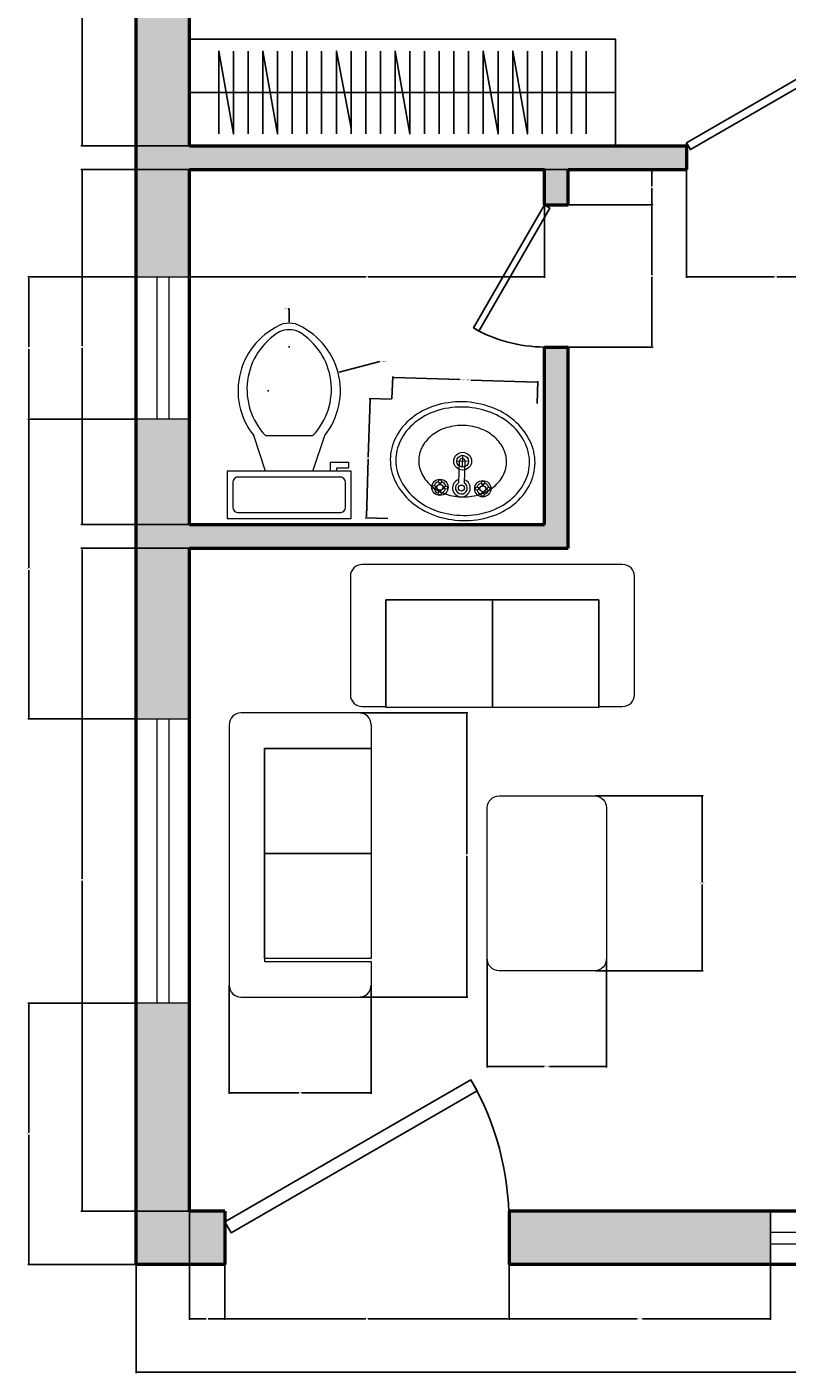
# Model space of a CAD drawing. Units: inches. Extents: x 2130 to 2425, y 2862 to 3216.
# Tile 1 of 4: x 2130 to 2259, y 2862 to 3089. Entities that reach past the tile are written whole.
import ezdxf

# ---------------------------------------------------------------- set-up
doc = ezdxf.new("R2010")
doc.units = ezdxf.units.IN
for name, color, linetype, lineweight in [('A-ANNO-DIMS', 2, 'Continuous', 18), ('A-DOOR', 3, 'Continuous', 25), ('A-FLOR-CASE', 9, 'Continuous', 25), ('A-FLOR-FIXT', 9, 'Continuous', 18), ('A-FURN', 8, 'Continuous', 18), ('A-GLAZ', 4, 'Continuous', 18), ('A-WALL', 7, 'Continuous', 50), ('A-WALL-PATT', 18, 'Continuous', 13)]:
    doc.layers.add(name, color=color, linetype=linetype, lineweight=lineweight)
doc.styles.get("Standard").update_dxf_attribs({"font": 'arial.ttf'})
doc.dimstyles.get("Standard").update_dxf_attribs({"dimtxt": 0.18, "dimasz": 0.18, "dimexe": 0.18, "dimexo": 0.0625, "dimgap": 0.09, "dimtad": 0, "dimtih": 1, "dimtoh": 1, "dimdec": 4, "dimzin": 0, "dimdsep": 46, "dimtxsty": 'Standard', "dimcen": 0.09, "dimadec": 0, "dimazin": 0, "dimtfac": 1, "dimtdec": 4, "dimtofl": 0, "dimtmove": 0, "dimatfit": 3, "dimfxl": 1, "dimtolj": 1, "dimtzin": 0, "dimarcsym": 0})

# ---------------------------------------------------------------- blocks, each defined once
blk = doc.blocks.new('Sink - Oval top')
for p, q in [((-1, 0), (1, 0)), ((0, 1), (0, -1))]:
    blk.add_line(p, q)
for points in [[(-12.23, 0.39, 0.117634), (-11.46, -3.36, 0.104469), (-8.88, -6.8, 0.090016), (-5.08, -9.07, 0.08192), (-0.32, -10.02, 0.08192), (4.49, -9.38, 0.090016), (8.42, -7.36, 0.104469), (11.22, -4.09, 0.117634), (12.23, -0.39, 0.117634), (11.46, 3.36, 0.104469), (8.88, 6.8, 0.090016), (5.08, 9.07, 0.08192), (0.32, 10.02, 0.08192), (-4.49, 9.38, 0.090016), (-8.42, 7.36, 0.104469), (-11.22, 4.09, 0.117634)], [(-11.29, 0.16, 0.118622), (-10.52, -3.25, 0.104678), (-8.07, -6.36, 0.089562), (-4.54, -8.37, 0.081185), (-0.13, -9.15, 0.081185), (4.3, -8.49, 0.089562), (7.89, -6.58, 0.104678), (10.42, -3.55, 0.118622), (11.29, -0.16, 0.118622), (10.52, 3.25, 0.104678), (8.07, 6.36, 0.089562), (4.54, 8.37, 0.081185), (0.13, 9.15, 0.081185), (-4.3, 8.49, 0.089562), (-7.89, 6.58, 0.104678), (-10.42, 3.55, 0.118622)], [(-7.42, 0.08, 0.118283), (-6.91, -2.17, 0.104607), (-5.29, -4.21, 0.089718), (-2.97, -5.53, 0.081436), (-0.07, -6.04, 0.081436), (2.84, -5.59, 0.089718), (5.2, -4.33, 0.104607), (6.86, -2.32, 0.118283), (7.42, -0.08, 0.118283), (6.91, 2.17, 0.104607), (5.29, 4.21, 0.089718), (2.97, 5.53, 0.081436), (0.07, 6.04, 0.081436), (-2.84, 5.59, 0.089718), (-5.2, 4.33, 0.104607), (-6.86, 2.32, 0.118283)]]:
    blk.add_lwpolyline(points, format="xyb", close=True)
for radius in [1.5, 1]:
    blk.add_circle((0, 0), radius)
blk = doc.blocks.new('Faucet - Bathroom top')
for p, q in [((-4.107, 0.125), (-4.375, 0.125)), ((-3.75, 0.4788), (-3.75, 0.75)), ((-3.5, 0.482), (-3.5, 0.75)), ((-3.1461, 0.125), (-2.875, 0.125)), ((3.143, 0.125), (2.875, 0.125)), ((3.5, 0.4788), (3.5, 0.75)), ((3.75, 0.482), (3.75, 0.75)), ((4.1039, 0.125), (4.375, 0.125)), ((-4.1039, -0.125), (-4.375, -0.125)), ((-3.75, -0.4821), (-3.75, -0.75)), ((-3.5, -0.4789), (-3.5, -0.75)), ((-3.143, -0.125), (-2.875, -0.125)), ((-0.5, -0.8639), (-0.5, -4.5)), ((0.5, -4.5), (0.5, -0.8631)), ((3.1461, -0.125), (2.875, -0.125)), ((3.5, -0.4821), (3.5, -0.75)), ((3.75, -0.4789), (3.75, -0.75)), ((4.107, -0.125), (4.375, -0.125))]:
    blk.add_line(p, q)
for centre, radius in [((-3.625, 0), 1.375), ((-4.625, 0), 0.2795), ((-3.625, 0), 0.5), ((-3.625, 1), 0.2795), ((-2.625, 0), 0.2795), ((0, 0), 0.5), ((3.625, 0), 1.375), ((2.625, 0), 0.2795), ((3.625, 0), 0.5), ((3.625, 1), 0.2795), ((4.625, 0), 0.2795), ((-3.625, -1), 0.2795), ((3.625, -1), 0.2795)]:
    blk.add_circle(centre, radius)
for centre, radius, start, end in [((-3.625, 0), 1, 105.2407, 164.2093), ((-3.625, 0), 1, 16.44125, 74.07887), ((0, 0), 1.5, 289.6514, 250.3603), ((0, 0), 1, 300.3431, 239.7554), ((3.625, 0), 1, 106.12, 164.0884), ((3.625, 0), 1, 16.23422, 73.90469), ((-3.625, 0), 1, 196.2342, 253.9047), ((-3.625, 0), 1, 286.12, 344.0884), ((3.625, 0), 1, 196.4413, 254.0789), ((3.625, 0), 1, 285.2407, 344.2093), ((0, -4.5), 0.5, 180, 0)]:
    blk.add_arc(centre, radius, start, end)
blk = doc.blocks.new('Toilet - top')
for p, q in [((9.5, -6), (9.5, -2)), ((-10, -8.5), (-8, -8.5)), ((-10, -9.5), (-10, -8.5)), ((-8, -8.5), (-8, -8)), ((-7, -8), (-7, -9.5)), ((-4, -8), (-6, -14)), ((4, -8), (6, -14)), ((-7, -9.5), (-10, -9.5)), ((4, -14), (-4, -14))]:
    blk.add_line(p, q)
blk.add_lwpolyline([(10.5, -8), (10.5, 0), (-10.5, 0), (-10.5, -8)], close=True)
for points in [[(-9.5, -2), (-9.5, -6)], [(8.5, -1), (-8.5, -1)], [(-8.5, -7), (8.5, -7)]]:
    blk.add_lwpolyline(points)
for centre, radius, start, end in [((-8.62, -1.88), 0.884, 81.8699, 188.1301), ((8.62, -1.88), 0.884, 351.8699, 98.1301), ((-8.62, -6.12), 0.884, 171.8699, 278.1301), ((8.62, -6.12), 0.884, 261.8699, 8.1301), ((3.52, -21.58), 12.17, 141.4691, 247.9714), ((4.2, -21.82), 11.33, 136.3677, 238.9468), ((-3.52, -21.58), 12.17, 292.0284, 38.5307), ((-4.2, -21.82), 11.33, 301.053, 43.6321), ((0, -27.88), 4, 245.7318, 294.2682), ((0, -29), 4, 254.8605, 285.1395)]:
    blk.add_arc(centre, radius, start, end)
blk = doc.blocks.new('*U10')
for p, q in [((0, 0), (0, -6)), ((40, 0), (40, -6))]:
    blk.add_line(p, q)
blk.add_lwpolyline([(0, 0), (34.64, 20), (35.52, 18.48), (0.87, -1.52)], close=True)
blk.add_arc((0, 0), 40, 0, 30)
blk = doc.blocks.new('*U11')
for p, q in [((0, 0), (0, 6)), ((40, 0), (40, 6))]:
    blk.add_line(p, q)
blk.add_lwpolyline([(0, 0), (34.64, -20), (35.52, -18.48), (0.87, 1.52)], close=True)
blk.add_arc((0, 0), 40, 330, 0)
blk = doc.blocks.new('WIN-48IN')
for p, q in [((0, 0), (0, 9)), ((48, 9), (48, 0)), ((0, 5.5), (48, 5.5)), ((0, 3.5), (48, 3.5))]:
    blk.add_line(p, q)
blk = doc.blocks.new('WARDROBE-72X18IN')
for p, q in [((0, 0), (0, 72)), ((0, 72), (18, 72)), ((9, 72), (9, 0)), ((18, 72), (18, 0)), ((2, 62.07), (16, 62.07)), ((2, 54.62), (16, 54.62)), ((2, 52.14), (16, 52.14)), ((2, 49.66), (16, 49.66)), ((2, 44.69), (16, 44.69)), ((2, 42.21), (16, 42.21)), ((2, 39.72), (16, 39.72)), ((2, 32.28), (16, 32.28)), ((2, 29.79), (16, 29.79)), ((2, 27.31), (16, 27.31)), ((2, 24.83), (16, 24.83)), ((2, 12.41), (16, 12.41)), ((2, 9.93), (16, 9.93)), ((2, 7.45), (16, 7.45)), ((2, 4.97), (16, 4.97)), ((18, 0), (0, 0))]:
    blk.add_line(p, q)
for points in [[(2, 67.03), (16, 67.03), (2, 64.55), (16, 64.55)], [(2, 59.59), (16, 59.59), (2, 57.1), (16, 57.1)], [(2, 47.17), (16, 47.17), (2.98, 44.69)], [(2, 37.24), (16, 37.24), (2, 34.76), (16, 34.76)], [(2, 22.35), (16, 22.35), (2, 19.86), (16, 19.86)], [(2, 17.38), (16, 17.38), (2, 14.9), (16, 14.9)]]:
    blk.add_lwpolyline(points)
blk.add_lwpolyline([(0, 0), (18, 0)], close=True)
blk = doc.blocks.new('*D23')
at = {"layer": 'A-ANNO-DIMS', "color": 0, "lineweight": -2, "transparency": 16777216}
for p, q in [((2191.77, 3026.18), (2191.89, 3029.98)), ((2192.07, 3029.8), (2203.22, 3029.44)), ((2216.25, 3029.02), (2205.09, 3029.38)), ((2216.31, 3025.39), (2216.43, 3029.19))]:
    blk.add_line(p, q, dxfattribs=at)
at = {"layer": 'A-ANNO-DIMS', "color": 0, "transparency": 16777216}
for points in [[(2192.07, 3029.83), (2192.07, 3029.77), (2191.89, 3029.8)], [(2216.25, 3029.05), (2216.24, 3028.99), (2216.43, 3029.01)]]:
    blk.add_solid(points, dxfattribs=at)
at = {"layer": 'Defpoints', "color": 0, "transparency": 16777216}
for p in [(2191.89, 3029.8), (2191.77, 3026.12), (2216.31, 3025.33)]:
    blk.add_point(p, dxfattribs=at)
at = {"layer": 'A-ANNO-DIMS', "color": 0, "transparency": 16777216, "insert": (2204.16, 3029.41), "char_height": 0.18, "attachment_point": 5}
blk.add_mtext('\\A1;BASIN 25 TYP.', dxfattribs=at)
blk = doc.blocks.new('*D24')
at = {"layer": 'A-ANNO-DIMS', "color": 0, "lineweight": -2, "transparency": 16777216}
for p, q in [((2188.08, 3026.06), (2187.77, 3016.36)), ((2191.71, 3026.12), (2187.91, 3026.25)), ((2187.45, 3006.29), (2187.76, 3015.99)), ((2191.06, 3006), (2187.26, 3006.12))]:
    blk.add_line(p, q, dxfattribs=at)
at = {"layer": 'A-ANNO-DIMS', "color": 0, "transparency": 16777216}
for points in [[(2188.05, 3026.06), (2188.11, 3026.06), (2188.09, 3026.24)], [(2187.42, 3006.29), (2187.48, 3006.29), (2187.44, 3006.11)]]:
    blk.add_solid(points, dxfattribs=at)
at = {"layer": 'Defpoints', "color": 0, "transparency": 16777216}
for p in [(2191.77, 3026.12), (2187.44, 3006.11), (2191.12, 3006)]:
    blk.add_point(p, dxfattribs=at)
at = {"layer": 'A-ANNO-DIMS', "color": 0, "transparency": 16777216, "insert": (2187.76, 3016.18), "char_height": 0.18, "attachment_point": 5}
blk.add_mtext('\\A1;20 TYP.', dxfattribs=at)
blk = doc.blocks.new('*D35')
at = {"layer": 'A-ANNO-DIMS', "color": 0, "lineweight": -2, "transparency": 16777216}
for p, q in [((2148.55, 2879.89), (2148.55, 2861.62)), ((2406.55, 2879.89), (2406.55, 2861.62)), ((2148.73, 2861.8), (2277.26, 2861.8)), ((2406.37, 2861.8), (2277.84, 2861.8))]:
    blk.add_line(p, q, dxfattribs=at)
at = {"layer": 'A-ANNO-DIMS', "color": 0, "transparency": 16777216}
for points in [[(2148.73, 2861.83), (2148.73, 2861.77), (2148.55, 2861.8)], [(2406.37, 2861.83), (2406.37, 2861.77), (2406.55, 2861.8)]]:
    blk.add_solid(points, dxfattribs=at)
at = {"layer": 'Defpoints', "color": 0, "transparency": 16777216}
for p in [(2148.55, 2879.95), (2406.55, 2879.95), (2406.55, 2861.8)]:
    blk.add_point(p, dxfattribs=at)
at = {"layer": 'A-ANNO-DIMS', "color": 0, "transparency": 16777216, "insert": (2277.55, 2861.8), "char_height": 0.18, "attachment_point": 5}
blk.add_mtext('\\A1;258', dxfattribs=at)
blk = doc.blocks.new('*D39')
at = {"layer": 'A-ANNO-DIMS', "color": 0, "lineweight": -2, "transparency": 16777216}
for p, q in [((2157.55, 2888.89), (2157.55, 2870.62)), ((2163.55, 2888.89), (2163.55, 2870.62)), ((2157.73, 2870.8), (2160.4, 2870.8)), ((2163.37, 2870.8), (2160.7, 2870.8))]:
    blk.add_line(p, q, dxfattribs=at)
at = {"layer": 'A-ANNO-DIMS', "color": 0, "transparency": 16777216}
for points in [[(2157.73, 2870.83), (2157.73, 2870.77), (2157.55, 2870.8)], [(2163.37, 2870.83), (2163.37, 2870.77), (2163.55, 2870.8)]]:
    blk.add_solid(points, dxfattribs=at)
at = {"layer": 'Defpoints', "color": 0, "transparency": 16777216}
for p in [(2157.55, 2888.95), (2163.55, 2888.95), (2157.55, 2870.8)]:
    blk.add_point(p, dxfattribs=at)
at = {"layer": 'A-ANNO-DIMS', "color": 0, "transparency": 16777216, "insert": (2160.55, 2870.8), "char_height": 0.18, "attachment_point": 5}
blk.add_mtext('\\A1;6', dxfattribs=at)
blk = doc.blocks.new('*D40')
at = {"layer": 'A-ANNO-DIMS', "color": 0, "lineweight": -2, "transparency": 16777216}
for p, q in [((2163.55, 2888.89), (2163.55, 2870.62)), ((2211.55, 2888.89), (2211.55, 2870.62)), ((2163.73, 2870.8), (2187.33, 2870.8)), ((2211.37, 2870.8), (2187.77, 2870.8))]:
    blk.add_line(p, q, dxfattribs=at)
at = {"layer": 'A-ANNO-DIMS', "color": 0, "transparency": 16777216}
for points in [[(2163.73, 2870.83), (2163.73, 2870.77), (2163.55, 2870.8)], [(2211.37, 2870.83), (2211.37, 2870.77), (2211.55, 2870.8)]]:
    blk.add_solid(points, dxfattribs=at)
at = {"layer": 'Defpoints', "color": 0, "transparency": 16777216}
for p in [(2163.55, 2888.95), (2211.55, 2888.95), (2163.55, 2870.8)]:
    blk.add_point(p, dxfattribs=at)
at = {"layer": 'A-ANNO-DIMS', "color": 0, "transparency": 16777216, "insert": (2187.55, 2870.8), "char_height": 0.18, "attachment_point": 5}
blk.add_mtext('\\A1;48', dxfattribs=at)
blk = doc.blocks.new('*D41')
at = {"layer": 'A-ANNO-DIMS', "color": 0, "lineweight": -2, "transparency": 16777216}
for p, q in [((2211.55, 2888.89), (2211.55, 2870.62)), ((2255.75, 2888.89), (2255.75, 2870.62)), ((2211.73, 2870.8), (2233.18, 2870.8)), ((2255.57, 2870.8), (2234.12, 2870.8))]:
    blk.add_line(p, q, dxfattribs=at)
at = {"layer": 'A-ANNO-DIMS', "color": 0, "transparency": 16777216}
for points in [[(2211.73, 2870.83), (2211.73, 2870.77), (2211.55, 2870.8)], [(2255.57, 2870.83), (2255.57, 2870.77), (2255.75, 2870.8)]]:
    blk.add_solid(points, dxfattribs=at)
at = {"layer": 'Defpoints', "color": 0, "transparency": 16777216}
for p in [(2211.55, 2888.95), (2255.75, 2888.95), (2211.55, 2870.8)]:
    blk.add_point(p, dxfattribs=at)
at = {"layer": 'A-ANNO-DIMS', "color": 0, "transparency": 16777216, "insert": (2233.65, 2870.8), "char_height": 0.18, "attachment_point": 5}
blk.add_mtext('\\A1;44.195', dxfattribs=at)
blk = doc.blocks.new('*D43')
at = {"layer": 'A-ANNO-DIMS', "color": 0, "lineweight": -2, "transparency": 16777216}
for p, q in [((2148.49, 2924.14), (2130.22, 2924.14)), ((2130.4, 2923.96), (2130.4, 2902.23)), ((2130.4, 2880.13), (2130.4, 2901.86)), ((2148.49, 2879.95), (2130.22, 2879.95))]:
    blk.add_line(p, q, dxfattribs=at)
at = {"layer": 'A-ANNO-DIMS', "color": 0, "transparency": 16777216}
for points in [[(2130.37, 2923.96), (2130.43, 2923.96), (2130.4, 2924.14)], [(2130.37, 2880.13), (2130.43, 2880.13), (2130.4, 2879.95)]]:
    blk.add_solid(points, dxfattribs=at)
at = {"layer": 'Defpoints', "color": 0, "transparency": 16777216}
for p in [(2130.4, 2924.14), (2148.55, 2924.14), (2148.55, 2879.95)]:
    blk.add_point(p, dxfattribs=at)
at = {"layer": 'A-ANNO-DIMS', "color": 0, "transparency": 16777216, "insert": (2130.4, 2902.05), "char_height": 0.18, "attachment_point": 5}
blk.add_mtext('\\A1;44.18', dxfattribs=at)
blk = doc.blocks.new('*D44')
at = {"layer": 'A-ANNO-DIMS', "color": 0, "lineweight": -2, "transparency": 16777216}
for p, q in [((2148.49, 3022.79), (2130.22, 3022.79)), ((2130.4, 3022.61), (2130.4, 2997.65)), ((2130.4, 2972.32), (2130.4, 2997.28)), ((2148.49, 2972.14), (2130.22, 2972.14))]:
    blk.add_line(p, q, dxfattribs=at)
at = {"layer": 'A-ANNO-DIMS', "color": 0, "transparency": 16777216}
for points in [[(2130.37, 3022.61), (2130.43, 3022.61), (2130.4, 3022.79)], [(2130.37, 2972.32), (2130.43, 2972.32), (2130.4, 2972.14)]]:
    blk.add_solid(points, dxfattribs=at)
at = {"layer": 'Defpoints', "color": 0, "transparency": 16777216}
for p in [(2130.4, 3022.79), (2148.55, 3022.79), (2148.55, 2972.14)]:
    blk.add_point(p, dxfattribs=at)
at = {"layer": 'A-ANNO-DIMS', "color": 0, "transparency": 16777216, "insert": (2130.4, 2997.46), "char_height": 0.18, "attachment_point": 5}
blk.add_mtext('\\A1;50.65', dxfattribs=at)
blk = doc.blocks.new('*D45')
at = {"layer": 'A-ANNO-DIMS', "color": 0, "lineweight": -2, "transparency": 16777216}
for p, q in [((2148.49, 3046.79), (2130.22, 3046.79)), ((2130.4, 3046.61), (2130.4, 3034.97)), ((2130.4, 3022.97), (2130.4, 3034.61)), ((2148.49, 3022.79), (2130.22, 3022.79))]:
    blk.add_line(p, q, dxfattribs=at)
at = {"layer": 'A-ANNO-DIMS', "color": 0, "transparency": 16777216}
for points in [[(2130.37, 3046.61), (2130.43, 3046.61), (2130.4, 3046.79)], [(2130.37, 3022.97), (2130.43, 3022.97), (2130.4, 3022.79)]]:
    blk.add_solid(points, dxfattribs=at)
at = {"layer": 'Defpoints', "color": 0, "transparency": 16777216}
for p in [(2130.4, 3046.79), (2148.55, 3046.79), (2148.55, 3022.79)]:
    blk.add_point(p, dxfattribs=at)
at = {"layer": 'A-ANNO-DIMS', "color": 0, "transparency": 16777216, "insert": (2130.4, 3034.79), "char_height": 0.18, "attachment_point": 5}
blk.add_mtext('\\A1;24', dxfattribs=at)
blk = doc.blocks.new('*D49')
at = {"layer": 'A-ANNO-DIMS', "color": 0, "lineweight": -2, "transparency": 16777216}
for p, q in [((2157.49, 3188.95), (2139.22, 3188.95)), ((2139.4, 3188.77), (2139.4, 3129.14)), ((2139.4, 3069.13), (2139.4, 3128.77)), ((2157.49, 3068.95), (2139.22, 3068.95))]:
    blk.add_line(p, q, dxfattribs=at)
at = {"layer": 'A-ANNO-DIMS', "color": 0, "transparency": 16777216}
for points in [[(2139.37, 3188.77), (2139.43, 3188.77), (2139.4, 3188.95)], [(2139.37, 3069.13), (2139.43, 3069.13), (2139.4, 3068.95)]]:
    blk.add_solid(points, dxfattribs=at)
at = {"layer": 'Defpoints', "color": 0, "transparency": 16777216}
for p in [(2139.4, 3188.95), (2157.55, 3188.95), (2157.55, 3068.95)]:
    blk.add_point(p, dxfattribs=at)
at = {"layer": 'A-ANNO-DIMS', "color": 0, "transparency": 16777216, "insert": (2139.4, 3128.95), "char_height": 0.18, "attachment_point": 5}
blk.add_mtext('\\A1;120', dxfattribs=at)
blk = doc.blocks.new('*D50')
at = {"layer": 'A-ANNO-DIMS', "color": 0, "lineweight": -2, "transparency": 16777216}
for p, q in [((2157.55, 3064.89), (2157.55, 3046.62)), ((2217.55, 3064.89), (2217.55, 3046.62)), ((2157.73, 3046.8), (2187.33, 3046.8)), ((2217.37, 3046.8), (2187.77, 3046.8))]:
    blk.add_line(p, q, dxfattribs=at)
at = {"layer": 'A-ANNO-DIMS', "color": 0, "transparency": 16777216}
for points in [[(2157.73, 3046.83), (2157.73, 3046.77), (2157.55, 3046.8)], [(2217.37, 3046.83), (2217.37, 3046.77), (2217.55, 3046.8)]]:
    blk.add_solid(points, dxfattribs=at)
at = {"layer": 'Defpoints', "color": 0, "transparency": 16777216}
for p in [(2157.55, 3064.95), (2217.55, 3064.95), (2157.55, 3046.8)]:
    blk.add_point(p, dxfattribs=at)
at = {"layer": 'A-ANNO-DIMS', "color": 0, "transparency": 16777216, "insert": (2187.55, 3046.8), "char_height": 0.18, "attachment_point": 5}
blk.add_mtext('\\A1;60', dxfattribs=at)
blk = doc.blocks.new('*D51')
at = {"layer": 'A-ANNO-DIMS', "color": 0, "lineweight": -2, "transparency": 16777216}
for p, q in [((2157.49, 3064.95), (2139.22, 3064.95)), ((2139.4, 3064.77), (2139.4, 3035.14)), ((2139.4, 3005.13), (2139.4, 3034.77)), ((2157.49, 3004.95), (2139.22, 3004.95))]:
    blk.add_line(p, q, dxfattribs=at)
at = {"layer": 'A-ANNO-DIMS', "color": 0, "transparency": 16777216}
for points in [[(2139.37, 3064.77), (2139.43, 3064.77), (2139.4, 3064.95)], [(2139.37, 3005.13), (2139.43, 3005.13), (2139.4, 3004.95)]]:
    blk.add_solid(points, dxfattribs=at)
at = {"layer": 'Defpoints', "color": 0, "transparency": 16777216}
for p in [(2139.4, 3064.95), (2157.55, 3064.95), (2157.55, 3004.95)]:
    blk.add_point(p, dxfattribs=at)
at = {"layer": 'A-ANNO-DIMS', "color": 0, "transparency": 16777216, "insert": (2139.4, 3034.95), "char_height": 0.18, "attachment_point": 5}
blk.add_mtext('\\A1;60', dxfattribs=at)
blk = doc.blocks.new('*D52')
at = {"layer": 'A-ANNO-DIMS', "color": 0, "lineweight": -2, "transparency": 16777216}
for p, q in [((2157.49, 3000.95), (2139.22, 3000.95)), ((2139.4, 3000.77), (2139.4, 2945.13)), ((2139.4, 2889.13), (2139.4, 2944.77)), ((2157.49, 2888.95), (2139.22, 2888.95))]:
    blk.add_line(p, q, dxfattribs=at)
at = {"layer": 'A-ANNO-DIMS', "color": 0, "transparency": 16777216}
for points in [[(2139.37, 3000.77), (2139.43, 3000.77), (2139.4, 3000.95)], [(2139.37, 2889.13), (2139.43, 2889.13), (2139.4, 2888.95)]]:
    blk.add_solid(points, dxfattribs=at)
at = {"layer": 'Defpoints', "color": 0, "transparency": 16777216}
for p in [(2139.4, 3000.95), (2157.55, 3000.95), (2157.55, 2888.95)]:
    blk.add_point(p, dxfattribs=at)
at = {"layer": 'A-ANNO-DIMS', "color": 0, "transparency": 16777216, "insert": (2139.4, 2944.95), "char_height": 0.18, "attachment_point": 5}
blk.add_mtext('\\A1;112', dxfattribs=at)
blk = doc.blocks.new('*D57')
at = {"layer": 'A-ANNO-DIMS', "color": 0, "lineweight": -2, "transparency": 16777216}
for p, q in [((2241.55, 3064.89), (2241.55, 3046.62)), ((2271.55, 3064.89), (2271.55, 3046.62)), ((2241.73, 3046.8), (2256.33, 3046.8)), ((2271.37, 3046.8), (2256.77, 3046.8))]:
    blk.add_line(p, q, dxfattribs=at)
at = {"layer": 'A-ANNO-DIMS', "color": 0, "transparency": 16777216}
for points in [[(2241.73, 3046.83), (2241.73, 3046.77), (2241.55, 3046.8)], [(2271.37, 3046.83), (2271.37, 3046.77), (2271.55, 3046.8)]]:
    blk.add_solid(points, dxfattribs=at)
at = {"layer": 'Defpoints', "color": 0, "transparency": 16777216}
for p in [(2241.55, 3064.95), (2271.55, 3064.95), (2241.55, 3046.8)]:
    blk.add_point(p, dxfattribs=at)
at = {"layer": 'A-ANNO-DIMS', "color": 0, "transparency": 16777216, "insert": (2256.55, 3046.8), "char_height": 0.18, "attachment_point": 5}
blk.add_mtext('\\A1;30', dxfattribs=at)
blk = doc.blocks.new('*D61')
at = {"layer": 'A-ANNO-DIMS', "color": 0, "lineweight": -2, "transparency": 16777216}
for p, q in [((2217.61, 3058.95), (2235.88, 3058.95)), ((2235.7, 3058.77), (2235.7, 3047.13)), ((2235.7, 3035.13), (2235.7, 3046.77)), ((2217.61, 3034.95), (2235.88, 3034.95))]:
    blk.add_line(p, q, dxfattribs=at)
at = {"layer": 'A-ANNO-DIMS', "color": 0, "transparency": 16777216}
for points in [[(2235.67, 3058.77), (2235.73, 3058.77), (2235.7, 3058.95)], [(2235.67, 3035.13), (2235.73, 3035.13), (2235.7, 3034.95)]]:
    blk.add_solid(points, dxfattribs=at)
at = {"layer": 'Defpoints', "color": 0, "transparency": 16777216}
for p in [(2217.55, 3058.95), (2217.55, 3034.95), (2235.7, 3034.95)]:
    blk.add_point(p, dxfattribs=at)
at = {"layer": 'A-ANNO-DIMS', "color": 0, "transparency": 16777216, "insert": (2235.7, 3046.95), "char_height": 0.18, "attachment_point": 5}
blk.add_mtext('\\A1;24', dxfattribs=at)
blk = doc.blocks.new('*D62')
at = {"layer": 'A-ANNO-DIMS', "color": 0, "lineweight": -2, "transparency": 16777216}
for p, q in [((2217.61, 3064.95), (2235.88, 3064.95)), ((2235.7, 3064.77), (2235.7, 3062.14)), ((2235.7, 3059.13), (2235.7, 3061.77)), ((2217.61, 3058.95), (2235.88, 3058.95))]:
    blk.add_line(p, q, dxfattribs=at)
at = {"layer": 'A-ANNO-DIMS', "color": 0, "transparency": 16777216}
for points in [[(2235.67, 3064.77), (2235.73, 3064.77), (2235.7, 3064.95)], [(2235.67, 3059.13), (2235.73, 3059.13), (2235.7, 3058.95)]]:
    blk.add_solid(points, dxfattribs=at)
at = {"layer": 'Defpoints', "color": 0, "transparency": 16777216}
for p in [(2217.55, 3064.95), (2217.55, 3058.95), (2235.7, 3058.95)]:
    blk.add_point(p, dxfattribs=at)
at = {"layer": 'A-ANNO-DIMS', "color": 0, "transparency": 16777216, "insert": (2235.7, 3061.95), "char_height": 0.18, "attachment_point": 5}
blk.add_mtext('\\A1;6', dxfattribs=at)
blk = doc.blocks.new('*D67')
at = {"layer": 'A-ANNO-DIMS', "color": 0, "lineweight": -2, "transparency": 16777216}
for p, q in [((2186.32, 2973.14), (2204.59, 2973.14)), ((2204.41, 2972.96), (2204.41, 2949.33)), ((2204.41, 2925.32), (2204.41, 2948.96)), ((2186.32, 2925.14), (2204.59, 2925.14))]:
    blk.add_line(p, q, dxfattribs=at)
at = {"layer": 'A-ANNO-DIMS', "color": 0, "transparency": 16777216}
for points in [[(2204.38, 2972.96), (2204.44, 2972.96), (2204.41, 2973.14)], [(2204.38, 2925.32), (2204.44, 2925.32), (2204.41, 2925.14)]]:
    blk.add_solid(points, dxfattribs=at)
at = {"layer": 'Defpoints', "color": 0, "transparency": 16777216}
for p in [(2186.26, 2973.14), (2186.26, 2925.14), (2204.41, 2925.14)]:
    blk.add_point(p, dxfattribs=at)
at = {"layer": 'A-ANNO-DIMS', "color": 0, "transparency": 16777216, "insert": (2204.41, 2949.14), "char_height": 0.18, "attachment_point": 5}
blk.add_mtext('\\A1;48', dxfattribs=at)
blk = doc.blocks.new('*D68')
at = {"layer": 'A-ANNO-DIMS', "color": 0, "lineweight": -2, "transparency": 16777216}
for p, q in [((2164.26, 2927.08), (2164.26, 2908.81)), ((2188.26, 2927.08), (2188.26, 2908.81)), ((2164.44, 2908.99), (2176.04, 2908.99)), ((2188.08, 2908.99), (2176.48, 2908.99))]:
    blk.add_line(p, q, dxfattribs=at)
at = {"layer": 'A-ANNO-DIMS', "color": 0, "transparency": 16777216}
for points in [[(2164.44, 2909.02), (2164.44, 2908.96), (2164.26, 2908.99)], [(2188.08, 2909.02), (2188.08, 2908.96), (2188.26, 2908.99)]]:
    blk.add_solid(points, dxfattribs=at)
at = {"layer": 'Defpoints', "color": 0, "transparency": 16777216}
for p in [(2164.26, 2927.14), (2188.26, 2927.14), (2164.26, 2908.99)]:
    blk.add_point(p, dxfattribs=at)
at = {"layer": 'A-ANNO-DIMS', "color": 0, "transparency": 16777216, "insert": (2176.26, 2908.99), "char_height": 0.18, "attachment_point": 5}
blk.add_mtext('\\A1;24', dxfattribs=at)
blk = doc.blocks.new('*D69')
at = {"layer": 'A-ANNO-DIMS', "color": 0, "lineweight": -2, "transparency": 16777216}
for p, q in [((2207.87, 2931.53), (2207.87, 2913.26)), ((2228.02, 2931.53), (2228.02, 2913.26)), ((2208.05, 2913.44), (2217.48, 2913.44)), ((2227.84, 2913.44), (2218.41, 2913.44))]:
    blk.add_line(p, q, dxfattribs=at)
at = {"layer": 'A-ANNO-DIMS', "color": 0, "transparency": 16777216}
for points in [[(2208.05, 2913.47), (2208.05, 2913.41), (2207.87, 2913.44)], [(2227.84, 2913.47), (2227.84, 2913.41), (2228.02, 2913.44)]]:
    blk.add_solid(points, dxfattribs=at)
at = {"layer": 'Defpoints', "color": 0, "transparency": 16777216}
for p in [(2207.87, 2931.59), (2228.02, 2931.59), (2207.87, 2913.44)]:
    blk.add_point(p, dxfattribs=at)
at = {"layer": 'A-ANNO-DIMS', "color": 0, "transparency": 16777216, "insert": (2217.94, 2913.44), "char_height": 0.18, "attachment_point": 5}
blk.add_mtext('\\A1;20.148', dxfattribs=at)
blk = doc.blocks.new('*D70')
at = {"layer": 'A-ANNO-DIMS', "color": 0, "lineweight": -2, "transparency": 16777216}
for p, q in [((2226.08, 2959.13), (2244.35, 2959.13)), ((2244.17, 2958.95), (2244.17, 2944.54)), ((2244.17, 2929.77), (2244.17, 2944.18)), ((2226.08, 2929.59), (2244.35, 2929.59))]:
    blk.add_line(p, q, dxfattribs=at)
at = {"layer": 'A-ANNO-DIMS', "color": 0, "transparency": 16777216}
for points in [[(2244.14, 2958.95), (2244.2, 2958.95), (2244.17, 2959.13)], [(2244.14, 2929.77), (2244.2, 2929.77), (2244.17, 2929.59)]]:
    blk.add_solid(points, dxfattribs=at)
at = {"layer": 'Defpoints', "color": 0, "transparency": 16777216}
for p in [(2226.02, 2959.13), (2226.02, 2929.59), (2244.17, 2929.59)]:
    blk.add_point(p, dxfattribs=at)
at = {"layer": 'A-ANNO-DIMS', "color": 0, "transparency": 16777216, "insert": (2244.17, 2944.36), "char_height": 0.18, "attachment_point": 5}
blk.add_mtext('\\A1;29.535', dxfattribs=at)
blk = doc.blocks.new('*D74')
at = {"layer": 'A-ANNO-DIMS', "color": 0, "lineweight": -2, "transparency": 16777216}
for p, q in [((2189.72, 3032.52), (2182.83, 3030.71)), ((2170.79, 3027.57), (2170.97, 3027.57)), ((2170.88, 3027.48), (2170.88, 3027.66))]:
    blk.add_line(p, q, dxfattribs=at)
at = {"layer": 'A-ANNO-DIMS', "color": 0, "transparency": 16777216}
blk.add_solid([(2182.82, 3030.73), (2182.84, 3030.68), (2182.65, 3030.66)], dxfattribs=at)
at = {"layer": 'Defpoints', "color": 0, "transparency": 16777216}
for p in [(2182.65, 3030.66), (2170.88, 3027.57)]:
    blk.add_point(p, dxfattribs=at)
at = {"layer": 'A-ANNO-DIMS', "color": 0, "transparency": 16777216, "insert": (2190.39, 3032.52), "char_height": 0.18, "attachment_point": 5}
blk.add_mtext('\\A1;4X R12.17', dxfattribs=at)
blk = doc.blocks.new('*D76')
at = {"layer": 'A-ANNO-DIMS', "color": 0, "lineweight": -2, "transparency": 16777216}
for p, q in [((2174.22, 3041.39), (2174.4, 3041.39)), ((2174.4, 3041.39), (2174.4, 3039.17)), ((2174.31, 3034.99), (2174.49, 3034.99)), ((2174.4, 3034.9), (2174.4, 3035.08))]:
    blk.add_line(p, q, dxfattribs=at)
at = {"layer": 'A-ANNO-DIMS', "color": 0, "transparency": 16777216}
blk.add_solid([(2174.43, 3039.17), (2174.37, 3039.17), (2174.4, 3038.99)], dxfattribs=at)
at = {"layer": 'Defpoints', "color": 0, "transparency": 16777216}
for p in [(2174.4, 3038.99), (2174.4, 3034.99)]:
    blk.add_point(p, dxfattribs=at)
at = {"layer": 'A-ANNO-DIMS', "color": 0, "transparency": 16777216, "insert": (2173.79, 3041.39), "char_height": 0.18, "attachment_point": 5}
blk.add_mtext('\\A1;4X R4', dxfattribs=at)

msp = doc.modelspace()

# ---------------------------------------------------------------- hatches: boundary and pattern name
at = {"layer": 'A-WALL-PATT'}
h = msp.add_hatch(color=256, dxfattribs=at)
h.dxf.hatch_style = 1
h.paths.add_polyline_path([(2186.3228, 3197.9544), (2148.5502, 3197.9544), (2148.5502, 3046.791), (2157.5502, 3046.791), (2157.5502, 3064.9544), (2217.5502, 3064.9544), (2217.5502, 3058.9544), (2221.1502, 3058.9544), (2221.5502, 3058.9544), (2221.5502, 3064.9544), (2241.5502, 3064.9544), (2241.5502, 3068.9544), (2157.5502, 3068.9544), (2157.5502, 3086.9544), (2157.5502, 3188.9544), (2186.3228, 3188.9544)])
h = msp.add_hatch(color=256, dxfattribs=at)
h.dxf.hatch_style = 1
h.paths.add_polyline_path([(2221.5502, 3034.9544), (2217.5502, 3034.9544), (2217.5502, 3004.9544), (2157.5502, 3004.9544), (2157.5502, 3022.791), (2148.5502, 3022.791), (2148.5502, 2972.1386), (2157.5502, 2972.1386), (2157.5502, 3000.9544), (2221.5502, 3000.9544)])
h = msp.add_hatch(color=256, dxfattribs=at)
h.dxf.hatch_style = 1
h.paths.add_polyline_path([(2163.5502, 2887.1544), (2163.5502, 2888.9544), (2157.5502, 2888.9544), (2157.5502, 2924.1386), (2148.5502, 2924.1386), (2148.5502, 2879.9544), (2163.5502, 2879.9544)])
h = msp.add_hatch(color=256, dxfattribs=at)
h.dxf.hatch_style = 1
h.paths.add_polyline_path([(2255.7452, 2888.9544), (2211.5502, 2888.9544), (2211.5502, 2879.9544), (2255.7452, 2879.9544)])

# ---------------------------------------------------------------- linework, layer by layer
at = {"layer": 'A-FURN'}
for p, q in [((2230.7457, 2998.2192), (2186.7457, 2998.2192)), ((2184.7457, 2996.2192), (2184.7457, 2976.2192)), ((2232.7457, 2976.2192), (2232.7457, 2996.2192)), ((2190.7457, 2992.2192), (2190.7457, 2974.2192)), ((2226.7457, 2992.2192), (2190.7457, 2992.2192)), ((2226.7457, 2974.2192), (2226.7457, 2992.2192)), ((2186.2568, 2973.1449), (2166.2568, 2973.1449)), ((2186.7457, 2974.2192), (2190.7457, 2974.2192)), ((2226.7457, 2974.2192), (2230.7457, 2974.2192)), ((2164.2568, 2971.1449), (2164.2568, 2927.1449)), ((2188.2568, 2971.1449), (2188.2568, 2967.1449)), ((2188.2568, 2967.1449), (2170.2568, 2967.1449)), ((2170.2568, 2967.1449), (2170.2568, 2931.1449)), ((2170.2568, 2931.1449), (2188.2568, 2931.1449)), ((2188.2568, 2931.1449), (2188.2568, 2927.1449)), ((2166.2568, 2925.1449), (2186.2568, 2925.1449))]:
    msp.add_line(p, q, dxfattribs=at)
for points in [[(2190.7457, 2992.2192), (2208.7457, 2992.2192), (2208.7457, 2974.0728), (2190.7457, 2974.0728)], [(2208.7457, 2992.2192), (2226.7457, 2992.2192), (2226.7457, 2974.0728), (2208.7457, 2974.0728)], [(2170.2568, 2967.1449), (2188.2568, 2967.1449), (2188.2568, 2949.3941), (2170.2568, 2949.3941)], [(2170.2568, 2949.3941), (2188.2568, 2949.3941), (2188.2568, 2931.6433), (2170.2568, 2931.6433)]]:
    msp.add_lwpolyline(points, close=True, dxfattribs=at)
msp.add_lwpolyline([(2209.8678, 2959.1295), (2226.0156, 2959.1295, -0.41421356), (2228.0156, 2957.1295), (2228.0156, 2931.5948, -0.41421356), (2226.0156, 2929.5948), (2209.8678, 2929.5948, -0.41421356), (2207.8678, 2931.5948), (2207.8678, 2957.1295, -0.41421356)], format="xyb", close=True, dxfattribs=at)
for centre, start, end in [((2186.7457, 2996.2192), 90, 180), ((2230.7457, 2996.2192), 0, 90), ((2186.7457, 2976.2192), 180, 270), ((2230.7457, 2976.2192), 270, 0), ((2166.2568, 2971.1449), 90, 180), ((2186.2568, 2971.1449), 0, 90), ((2166.2568, 2927.1449), 180, 270), ((2186.2568, 2927.1449), 270, 0)]:
    msp.add_arc(centre, 2, start, end, dxfattribs=at)
at = {"layer": 'A-GLAZ'}
for p, q in [((2148.5502, 3046.791), (2157.5502, 3046.791)), ((2152.0502, 3046.791), (2152.0502, 3022.791)), ((2154.0502, 3046.791), (2154.0502, 3022.791)), ((2157.5502, 3022.791), (2148.5502, 3022.791))]:
    msp.add_line(p, q, dxfattribs=at)
at = {"layer": 'A-WALL'}
for p, q in [((2157.5502, 3068.9544), (2157.5502, 3188.9544)), ((2157.5502, 3068.9544), (2241.5502, 3068.9544)), ((2241.5502, 3068.9544), (2241.5502, 3064.9544)), ((2157.5502, 3064.9544), (2217.5502, 3064.9544)), ((2157.5502, 3004.9544), (2157.5502, 3064.9544)), ((2217.5502, 3058.9544), (2217.5502, 3064.9544)), ((2221.5502, 3064.9544), (2241.5502, 3064.9544)), ((2221.5502, 3058.9544), (2221.5502, 3064.9544)), ((2217.5502, 3058.9544), (2221.5502, 3058.9544)), ((2217.5502, 3004.9544), (2217.5502, 3034.9544)), ((2217.5502, 3034.9544), (2221.5502, 3034.9544)), ((2221.5502, 3000.9544), (2221.5502, 3034.9544)), ((2157.5502, 3004.9544), (2217.5502, 3004.9544)), ((2157.5502, 2888.9544), (2157.5502, 3000.9544)), ((2157.5502, 3000.9544), (2221.5502, 3000.9544)), ((2163.5502, 2888.9544), (2157.5502, 2888.9544)), ((2163.5502, 2888.9544), (2163.5502, 2879.9544)), ((2323.5502, 2888.9544), (2211.5502, 2888.9544)), ((2211.5502, 2888.9544), (2211.5502, 2879.9544))]:
    msp.add_line(p, q, dxfattribs=at)
msp.add_lwpolyline([(2163.5502, 2879.9544), (2148.5502, 2879.9544), (2148.5502, 3197.9544), (2406.5502, 3197.9544), (2406.5502, 2879.9544), (2211.5502, 2879.9544)], dxfattribs=at)

# ---------------------------------------------------------------- block references
at = {"layer": 'A-DOOR'}
for p, xscale, yscale, zscale in [((2241.5502, 3069.4544), 0.75, 0.75, 0.75), ((2163.5502, 2887.1544), 1.199999999999999, 1.199999999999999, 1.199999999999999)]:
    msp.add_blockref('*U10', p, dxfattribs=dict(at, xscale=xscale, yscale=yscale, zscale=zscale))
at = {"layer": 'A-DOOR', "xscale": 0.6, "yscale": 0.6, "zscale": 0.6, "rotation": 270}
msp.add_blockref('*U11', (2217.5502, 3058.9544), dxfattribs=at)
at = {"layer": 'A-FLOR-CASE', "rotation": 90.0000000000085}
msp.add_blockref('WARDROBE-72X18IN', (2229.5506, 3068.9542), dxfattribs=at)
at = {"layer": 'A-FLOR-FIXT'}
for name, p, rotation in [('Toilet - top', (2174.4045, 3005.9873), 180), ('Sink - Oval top', (2203.7134, 3015.6629), 178.1544699151333), ('Faucet - Bathroom top', (2203.4996, 3011.1306), 178.1544699151333)]:
    msp.add_blockref(name, p, dxfattribs=dict(at, rotation=rotation))
at = {"layer": 'A-GLAZ', "rotation": 269.999999999997}
msp.add_blockref('WIN-48IN', (2148.5498, 2972.1384), dxfattribs=at)
at = {"layer": 'A-GLAZ'}
msp.add_blockref('WIN-48IN', (2255.7454, 2879.954), dxfattribs=at)

# ---------------------------------------------------------------- dimensions: what is measured, and where the dimension line sits
at = {"layer": 'A-ANNO-DIMS'}
for base, p1, p2, angle, override, picture, middle in [((2139.4002, 3188.9544), (2157.5502, 3068.9544), (2157.5502, 3188.9544), 90, {"dimdec": 0, "dimlfac": 1, "dimrnd": 0, "dimzin": 0, "dimdsep": 46, "dimlunit": 2}, '*D49', (2139.4002, 3128.9544)), ((2139.4002, 3064.9544), (2157.5502, 3004.9544), (2157.5502, 3064.9544), 90, {"dimdec": 0, "dimlfac": 1, "dimrnd": 0, "dimzin": 0, "dimdsep": 46, "dimlunit": 2}, '*D51', (2139.4002, 3034.9544)), ((2157.5502, 3046.8044), (2217.5502, 3064.9544), (2157.5502, 3064.9544), 180, {"dimdec": 0, "dimlfac": 1, "dimrnd": 0, "dimzin": 0, "dimdsep": 46, "dimlunit": 2}, '*D50', (2187.5502, 3046.8044)), ((2235.7002, 3058.9544), (2217.5502, 3064.9544), (2217.5502, 3058.9544), 270, {"dimdec": 0, "dimlfac": 1, "dimrnd": 0, "dimzin": 0, "dimdsep": 46, "dimlunit": 2}, '*D62', (2235.7002, 3061.9544)), ((2241.5502, 3046.8044), (2271.5502, 3064.9544), (2241.5502, 3064.9544), 180, {"dimdec": 0, "dimlfac": 1, "dimrnd": 0, "dimzin": 0, "dimdsep": 46, "dimlunit": 2}, '*D57', (2256.5502, 3046.8044)), ((2235.7002, 3034.9544), (2217.5502, 3058.9544), (2217.5502, 3034.9544), 270, {"dimdec": 0, "dimlfac": 1, "dimrnd": 0, "dimzin": 0, "dimdsep": 46, "dimlunit": 2}, '*D61', (2235.7002, 3046.9544)), ((2130.4002, 3046.791), (2148.5502, 3022.791), (2148.5502, 3046.791), 90, {"dimdec": 0, "dimlfac": 1, "dimrnd": 0, "dimzin": 0, "dimdsep": 46, "dimlunit": 2}, '*D45', (2130.4002, 3034.791)), ((2130.4002, 3022.791), (2148.5502, 2972.1386), (2148.5502, 3022.791), 90, {"dimdec": 2, "dimlfac": 1, "dimrnd": 0, "dimzin": 0, "dimdsep": 46, "dimlunit": 2}, '*D44', (2130.4002, 2997.4648)), ((2139.4002, 3000.9544), (2157.5502, 2888.9544), (2157.5502, 3000.9544), 90, {"dimdec": 0, "dimlfac": 1, "dimrnd": 0, "dimzin": 0, "dimdsep": 46, "dimlunit": 2}, '*D52', (2139.4002, 2944.9544)), ((2204.4068, 2925.1449), (2186.2568, 2973.1449), (2186.2568, 2925.1449), 270, {"dimdec": 0, "dimlfac": 1, "dimrnd": 0, "dimzin": 0, "dimdsep": 46, "dimlunit": 2}, '*D67', (2204.4068, 2949.1449)), ((2244.1656, 2929.5948), (2226.0156, 2959.1295), (2226.0156, 2929.5948), 270, {"dimdec": 3, "dimlfac": 1, "dimrnd": 0, "dimzin": 0, "dimdsep": 46, "dimlunit": 2}, '*D70', (2244.1656, 2944.3622)), ((2207.8678, 2913.4448), (2228.0156, 2931.5948), (2207.8678, 2931.5948), 180, {"dimdec": 3, "dimlfac": 1, "dimrnd": 0, "dimzin": 0, "dimdsep": 46, "dimlunit": 2}, '*D69', (2217.9417, 2913.4448)), ((2164.2568, 2908.9949), (2188.2568, 2927.1449), (2164.2568, 2927.1449), 180, {"dimdec": 0, "dimlfac": 1, "dimrnd": 0, "dimzin": 0, "dimdsep": 46, "dimlunit": 2}, '*D68', (2176.2568, 2908.9949)), ((2130.4002, 2924.1386), (2148.5502, 2879.9544), (2148.5502, 2924.1386), 90, {"dimdec": 2, "dimlfac": 1, "dimrnd": 0, "dimzin": 0, "dimdsep": 46, "dimlunit": 2}, '*D43', (2130.4002, 2902.0465)), ((2157.5502, 2870.8044), (2163.5502, 2888.9544), (2157.5502, 2888.9544), 180, {"dimdec": 0, "dimlfac": 1, "dimrnd": 0, "dimzin": 0, "dimdsep": 46, "dimlunit": 2}, '*D39', (2160.5502, 2870.8044)), ((2163.5502, 2870.8044), (2211.5502, 2888.9544), (2163.5502, 2888.9544), 180, {"dimdec": 0, "dimlfac": 1, "dimrnd": 0, "dimzin": 0, "dimdsep": 46, "dimlunit": 2}, '*D40', (2187.5502, 2870.8044)), ((2211.5502, 2870.8044), (2255.7452, 2888.9544), (2211.5502, 2888.9544), 180, {"dimdec": 3, "dimlfac": 1, "dimrnd": 0, "dimzin": 0, "dimdsep": 46, "dimlunit": 2}, '*D41', (2233.6477, 2870.8044))]:
    dim = msp.add_linear_dim(base=base, p1=p1, p2=p2, angle=angle, dimstyle='Standard', override=override, dxfattribs=at)
    dim.commit()
    dim.dimension.update_dxf_attribs({"geometry": picture, "text_midpoint": middle})
for center, mpoint, override, picture, middle in [((2174.4045, 3034.9873), (2174.404, 3038.9873), {"dimdec": 0, "dimlfac": 1, "dimrnd": 0, "dimzin": 0, "dimdsep": 46, "dimlunit": 2}, '*D76', (2173.7919, 3041.3873)), ((2170.885, 3027.5678), (2182.6546, 3030.6599), {"dimdec": 2, "dimlfac": 1, "dimrnd": 0, "dimzin": 0, "dimdsep": 46, "dimlunit": 2}, '*D74', (2189.7163, 3032.5151))]:
    dim = msp.add_radius_dim(center=center, mpoint=mpoint, text='4X <>', dimstyle='Standard', override=override, dxfattribs=at)
    dim.commit()
    dim.dimension.update_dxf_attribs({"geometry": picture, "text_midpoint": middle, "dimtype": 164})
for base, p1, p2, angle, text, picture, middle in [((2191.8872, 3029.802), (2216.3067, 3025.3306), (2191.7686, 3026.1213), 178.15447, 'BASIN <> TYP.', '*D23', (2204.1562, 3029.4067)), ((2187.4393, 3006.1138), (2191.7686, 3026.1213), (2191.1201, 3005.9952), 268.15447, '<> TYP.', '*D24', (2187.7636, 3016.1768))]:
    dim = msp.add_linear_dim(base=base, p1=p1, p2=p2, angle=angle, text=text, dimstyle='Standard', override={"dimdec": 0, "dimlfac": 1, "dimrnd": 0, "dimzin": 0, "dimdsep": 46, "dimlunit": 2}, dxfattribs=at)
    dim.commit()
    dim.dimension.update_dxf_attribs({"geometry": picture, "text_midpoint": middle})
dim = msp.add_linear_dim(base=(2406.5502, 2861.8044), p1=(2148.5502, 2879.9544), p2=(2406.5502, 2879.9544), dimstyle='Standard', override={"dimdec": 0, "dimlfac": 1, "dimrnd": 0, "dimzin": 0, "dimdsep": 46, "dimlunit": 2}, dxfattribs=at)
dim.commit()
dim.dimension.update_dxf_attribs({"geometry": '*D35', "text_midpoint": (2277.5502, 2861.8044)})

doc.saveas('drawing.dxf')
